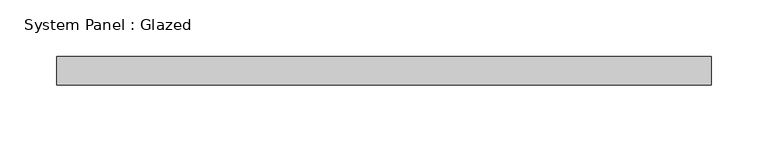
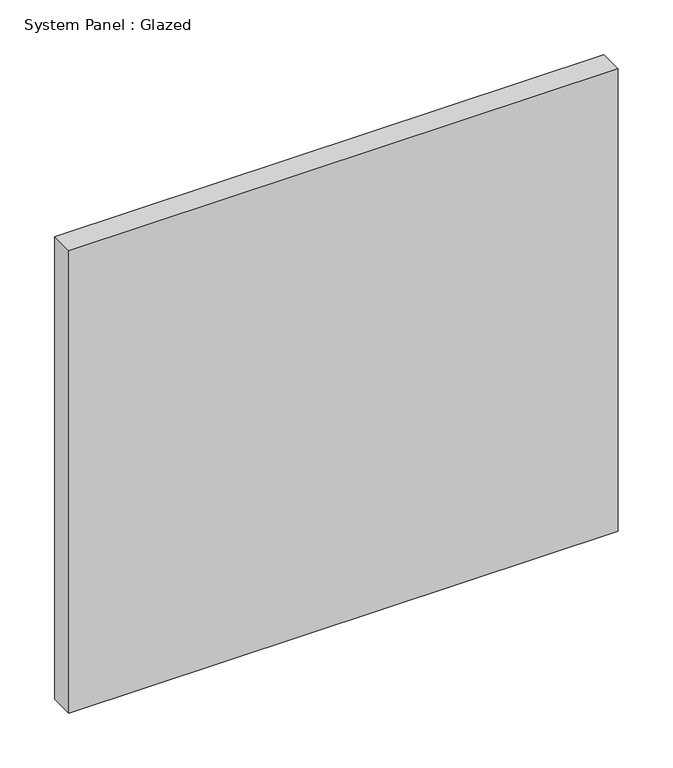
"""IFC4 building model written with IfcOpenShell, lengths in millimetres: plate geometry, System Panel : Glazed."""

from ifc_helpers import new_model, si_unit, origin, origin_with_axes, place, context, project, spatial, polyline, outline, extrude, source, transform, mapped, element, save


def system_panel_glazed_3760a879(model_context):
    return source(origin(), model_context, "Body", "SweptSolid", [
        extrude(outline(polyline([(288.925, -44.45), (-288.925, -44.45), (-288.925, -19.05), (288.925, -19.05), (288.925, -44.45)])), origin_with_axes(), (0.0, 0.0, 1.0), 514.35),
    ])


if __name__ == "__main__":
    model = new_model("IFC4")
    model_context = context("Model", 3, world=origin())
    ifc_project = project(units=[si_unit("LENGTHUNIT", "METRE", prefix="MILLI")], contexts=[model_context])
    site = spatial("IfcSite", under=ifc_project)
    building = spatial("IfcBuilding", under=site)
    placement = place(None, origin())
    system_panel_glazed_shape = system_panel_glazed_3760a879(model_context)
    element("IfcPlate", 1, ObjectType="System Panel : Glazed", at=placement, inside=building, context=model_context, shape_type="MappedRepresentation", body=[
        mapped(system_panel_glazed_shape, transform((0.0, 0.0, 0.0), x_axis=(1.0, 0.0, 0.0), y_axis=(0.0, 1.0, 0.0), z_axis=(0.0, 0.0, 1.0))),
    ])
    save(model, "model.ifc")

# Revit data of these elements
# Type "System Panel : Glazed"
#   Construction Type Id = "GSP4R"
#   Analytic Construction = "1/8 in Pilkington single glazing"
#   Visual Light Transmittance = 0.9
#   Solar Heat Gain Coefficient = 0.86
#   Heat Transfer Coefficient (U) = 1.18115 BTU/(h·ft²·°F)
# Element 1 (IfcPlate, "System Panel : Glazed")
#   Materials on its faces: "Glass"
# Materials
#   "Glass": class "Glass", colour RGB 0 128 192, transparency 0.75, Description = "Soda Lime Glass", Cost = 0
